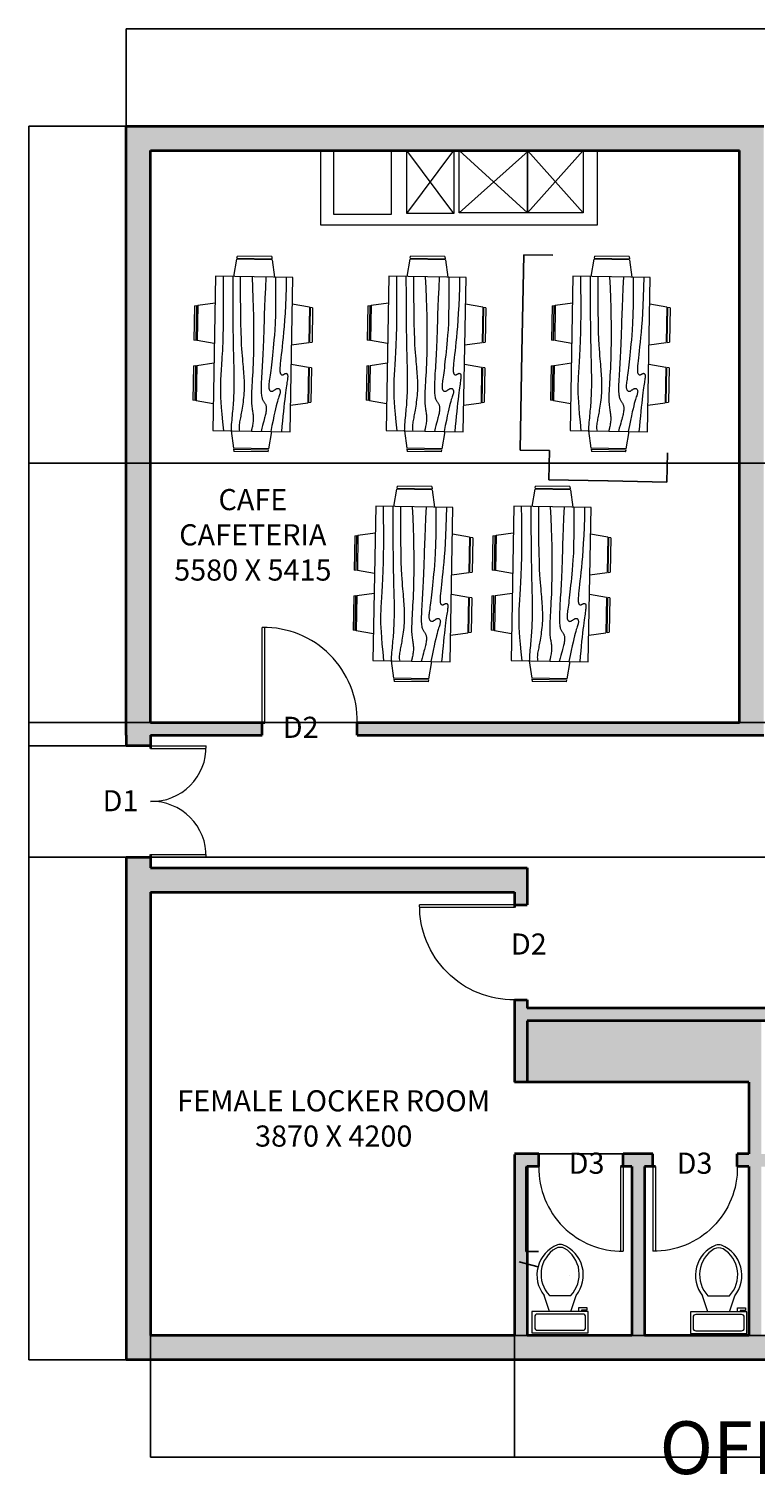
# Model space of a CAD drawing. Units: millimetres. Extents: x 14737 to 34075, y 1723 to 15415.
# Tile 1 of 2: x 14737 to 21616, y 1723 to 15415. Entities that reach past the tile are written whole.
import ezdxf

# ---------------------------------------------------------------- set-up
doc = ezdxf.new("R2010")
doc.units = ezdxf.units.MM
doc.header["$PDMODE"] = 32
doc.header["$PDSIZE"] = 100
for name, color, linetype, lineweight in [('A-ANNO-DIMS', 2, 'Continuous', 18), ('A-ANNO-TITL', 7, 'Continuous', 35), ('A-AREA-IDEN', 7, 'Continuous', 25), ('A-DOOR', 4, 'Continuous', 18), ('A-DOOR-IDEN', 3, 'Continuous', 18), ('A-EQPM', 8, 'Continuous', 18), ('A-FLOR-FIXT', 9, 'Continuous', 18), ('A-FURN', 8, 'Continuous', 18), ('A-WALL', 7, 'Continuous', 35), ('A-WALL-PATT', 252, 'Continuous', 13)]:
    doc.layers.add(name, color=color, linetype=linetype, lineweight=lineweight)
doc.styles.get("Standard").update_dxf_attribs({"font": 'arial.ttf'})
doc.dimstyles.get("Standard").update_dxf_attribs({"dimtxt": 0.18, "dimasz": 0.18, "dimexe": 0.18, "dimexo": 0.0625, "dimgap": 0.09, "dimtad": 0, "dimtih": 1, "dimtoh": 1, "dimdec": 4, "dimzin": 0, "dimdsep": 46, "dimtxsty": 'Standard', "dimcen": 0.09, "dimadec": 0, "dimazin": 0, "dimtfac": 1, "dimtdec": 4, "dimtofl": 0, "dimtmove": 0, "dimatfit": 3, "dimfxl": 1, "dimtolj": 1, "dimtzin": 0, "dimarcsym": 0})

# ---------------------------------------------------------------- blocks, each defined once
blk = doc.blocks.new('Dining Set - 36 x 72 in.')
for p, q in [((-22, 27.5), (-22.15620000000001, 26.50042)), ((-22, 27.5), (-6, 27.5)), ((-5.843700000000012, 26.49966), (-6, 27.5)), ((6, 27.5), (5.843799999999987, 26.50042)), ((6, 27.5), (22, 27.5)), ((22.15629999999999, 26.49966), (22, 27.5)), ((-22.23430000000002, 26.00059), (-23.48470000000003, 17.99762)), ((-22.23040000000003, 26), (-5.760800000000017, 26)), ((-5.841600000000028, 26.5), (-22.15340000000003, 26.5)), ((-4.515199999999992, 17.99762), (-5.765500000000031, 25.99926)), ((5.765699999999981, 26.00059), (4.515299999999967, 17.99762)), ((5.769599999999968, 26), (22.23919999999998, 26)), ((22.15839999999997, 26.5), (5.846599999999966, 26.5)), ((23.48480000000001, 17.99762), (22.23449999999997, 25.99926)), ((36, 18), (-36, 18)), ((-36, 18), (-36, -18)), ((36, -18), (36, 18)), ((-45.49999999999999, 8.000000000000004), (-44.50040000000001, 8.156170000000007)), ((-45.49999999999999, 8.000000000000004), (-45.49999999999999, -7.999999999999996)), ((-44.5, -8.15843), (-44.5, 8.153380000000002)), ((-44.00060000000002, 8.234280000000002), (-35.99760000000003, 9.484740000000006)), ((-44, 8.230410000000003), (-44, -8.239149999999999)), ((44.00059999999996, 8.234280000000002), (35.99759999999998, 9.484740000000006)), ((44, 8.230410000000003), (44, -8.239149999999999)), ((44.5, -8.15843), (44.5, 8.153380000000002)), ((45.49999999999999, 8.000000000000004), (44.50049999999999, 8.156170000000007)), ((45.49999999999999, 8.000000000000004), (45.49999999999999, -7.999999999999996)), ((-44.49970000000002, -8.156309999999994), (-45.49999999999999, -7.999999999999996)), ((-35.99760000000003, -9.484759999999998), (-43.9993, -8.234499999999993)), ((35.99759999999998, -9.484759999999998), (43.9993, -8.234499999999993)), ((44.49969999999995, -8.156309999999994), (45.49999999999999, -7.999999999999996)), ((-36, -18), (36, -18)), ((-22.23430000000002, -26.0006), (-23.48470000000003, -17.99762)), ((-4.515199999999992, -17.99762), (-5.765500000000031, -25.99928)), ((5.765699999999981, -26.0006), (4.515299999999967, -17.99762)), ((23.48480000000001, -17.99762), (22.23449999999997, -25.99928)), ((-22.23040000000003, -26), (-5.760800000000017, -26)), ((-22, -27.5), (-22.15620000000001, -26.50044)), ((-5.841600000000028, -26.5), (-22.15340000000003, -26.5)), ((-5.843700000000012, -26.49967), (-6, -27.5)), ((5.769599999999968, -26), (22.23919999999998, -26)), ((6, -27.5), (5.843799999999987, -26.50044)), ((22.15839999999997, -26.5), (5.846599999999966, -26.5)), ((22.15629999999999, -26.49967), (22, -27.5)), ((-22, -27.5), (-6, -27.5)), ((6, -27.5), (22, -27.5))]:
    blk.add_line(p, q)
for points in [[(-36, 15), (-31.17720000000003, 14.97754), (-26.80790000000002, 14.91406), (-22.85380000000003, 14.81543), (-19.27600000000001, 14.6875), (-16.03620000000001, 14.53613), (-13.09570000000002, 14.36718), (-10.41590000000002, 14.18652), (-7.958300000000008, 14), (-5.690400000000011, 13.81315), (-3.603499999999996, 13.63021), (-1.695400000000006, 13.45508), (0.0364999999999896, 13.29166), (1.594499999999982, 13.14388), (2.981099999999969, 13.01562), (4.198800000000005, 12.9108), (5.25, 12.83333), (6.139299999999991, 12.78613), (6.880200000000002, 12.76823), (7.488299999999981, 12.77767), (7.979199999999991, 12.8125), (8.368499999999983, 12.87077), (8.671899999999994, 12.95052), (8.904899999999998, 13.0498), (9.083300000000008, 13.16666), (9.220499999999959, 13.29899000000001), (9.32159999999999, 13.44401), (9.389499999999998, 13.59879), (9.427099999999996, 13.76041), (9.437299999999993, 13.92594), (9.423200000000008, 14.09245), (9.387499999999989, 14.257), (9.333300000000008, 14.41666), (9.263800000000003, 14.56917), (9.183600000000013, 14.71484), (9.097499999999968, 14.85465), (9.010400000000004, 14.98958), (8.92719999999997, 15.12060000000001), (8.852899999999975, 15.2487), (8.79219999999998, 15.37483), (8.75, 15.5), (8.730500000000006, 15.62467), (8.734399999999994, 15.74739), (8.761699999999962, 15.86621), (8.8125, 15.97916), (8.886699999999962, 16.08431), (8.984399999999994, 16.17968), (9.105500000000006, 16.26334), (9.25, 16.33333), (9.418900000000008, 16.38802), (9.617199999999968, 16.42708), (9.850599999999986, 16.45052), (10.125, 16.45833), (10.44630000000001, 16.45052), (10.82029999999997, 16.42708), (11.25290000000001, 16.38802), (11.75, 16.33333), (12.3184, 16.26318), (12.96940000000001, 16.17838), (13.7151, 16.07991), (14.5677, 15.96875), (15.53949999999997, 15.84586), (16.64259999999996, 15.71224), (17.88929999999999, 15.56884), (19.29169999999999, 15.41666), (20.85899999999998, 15.25667), (22.58789999999999, 15.08984), (24.47210000000001, 14.91715), (26.5052, 14.73958), (28.68090000000001, 14.5581), (30.99289999999996, 14.3737), (33.43469999999996, 14.18733), (36, 14)], [(-36, 10), (-28.97660000000002, 10.14274000000001), (-23.17250000000001, 10.20442), (-18.42410000000001, 10.19775), (-14.5677, 10.13541), (-11.43990000000002, 10.03011), (-8.87700000000001, 9.894530000000007), (-6.715399999999988, 9.741370000000005), (-4.791699999999991, 9.58333), (-2.96980000000002, 9.43082), (-1.224600000000009, 9.285150000000005), (0.4414999999999623, 9.14534), (2.02600000000001, 9.010410000000004), (3.526599999999973, 8.879390000000004), (4.940799999999967, 8.751300000000004), (6.265999999999962, 8.625160000000005), (7.5, 8.500000000000004), (8.641099999999994, 8.375490000000003), (9.691399999999987, 8.253900000000005), (10.65379999999999, 8.13818), (11.53120000000001, 8.031250000000004), (12.32669999999996, 7.936030000000005), (13.043, 7.85547), (13.68309999999997, 7.792480000000001), (14.25, 7.750000000000003), (14.74709999999999, 7.730300000000003), (15.17969999999997, 7.733070000000001), (15.55369999999999, 7.757320000000003), (15.875, 7.80208), (16.14940000000001, 7.866370000000006), (16.38279999999997, 7.94922), (16.58109999999999, 8.04964), (16.75, 8.166660000000004), (16.89439999999996, 8.29915), (17.01429999999999, 8.445310000000003), (17.1089, 8.603190000000001), (17.17709999999999, 8.77083), (17.21799999999996, 8.946290000000001), (17.2305, 9.127600000000005), (17.21369999999996, 9.312820000000006), (17.16669999999999, 9.500000000000004), (17.08949999999999, 9.687500000000004), (16.98699999999996, 9.875000000000004), (16.86489999999998, 10.0625), (16.72919999999999, 10.25), (16.5856, 10.4375), (16.44009999999997, 10.625), (16.29849999999999, 10.8125), (16.16669999999999, 11), (16.05000000000001, 11.18733), (15.95179999999999, 11.3737), (15.8752, 11.5581), (15.8229, 11.73958), (15.798, 11.91715), (15.80340000000001, 12.08984), (15.84199999999998, 12.25667), (15.91669999999999, 12.41666), (16.02949999999998, 12.56836), (16.17840000000001, 12.70833), (16.3605, 12.83268), (16.5729, 12.9375), (16.8127, 13.01888000000001), (17.07679999999999, 13.07291), (17.36250000000001, 13.0957), (17.66669999999999, 13.08333), (17.98939999999999, 13.03312), (18.34179999999998, 12.94726), (18.7382, 12.82918), (19.1927, 12.68229), (19.71949999999998, 12.51001), (20.33269999999999, 12.31575), (21.04649999999998, 12.10294), (21.875, 11.875), (22.83569999999997, 11.63354), (23.95900000000001, 11.37304), (25.27859999999999, 11.08618), (26.82819999999998, 10.76562), (28.64139999999998, 10.40405), (30.75200000000001, 9.994140000000005), (33.1936, 9.528560000000002), (36, 9.000000000000004)], [(-36, 5.500000000000003), (-30.71570000000003, 5.334800000000004), (-26.06900000000002, 5.20963), (-21.99459999999999, 5.11767), (-18.42709999999999, 5.05208), (-15.30090000000001, 5.006020000000003), (-12.55080000000004, 4.972650000000005), (-10.1112, 4.945150000000001), (-7.916699999999991, 4.916660000000003), (-5.908999999999991, 4.881670000000003), (-4.058600000000012, 4.839840000000005), (-2.342899999999985, 4.792150000000003), (-0.7395999999999959, 4.73958), (0.7738999999999692, 4.683100000000006), (2.21999999999997, 4.623700000000003), (3.621299999999962, 4.562330000000006), (5, 4.500000000000003), (6.37299999999999, 4.437820000000005), (7.734399999999993, 4.377600000000004), (9.072299999999984, 4.321290000000001), (10.375, 4.27083), (11.63089999999999, 4.228190000000001), (12.8281, 4.195310000000002), (13.95509999999996, 4.17415), (15, 4.166660000000003), (15.95400000000001, 4.174480000000006), (16.81899999999996, 4.197910000000003), (17.6001, 4.236980000000006), (18.30209999999999, 4.291660000000003), (18.92989999999997, 4.361980000000006), (19.48829999999998, 4.447910000000003), (19.98230000000001, 4.549480000000006), (20.41669999999999, 4.666660000000003), (20.79689999999999, 4.798990000000006), (21.1302, 4.944010000000002), (21.42449999999997, 5.098790000000004), (21.6875, 5.260410000000003), (21.92709999999999, 5.42594), (22.15109999999999, 5.592450000000003), (22.36719999999997, 5.757000000000001), (22.58339999999998, 5.916660000000003), (22.80649999999997, 6.068680000000004), (23.04039999999998, 6.210930000000001), (23.28789999999998, 6.341470000000004), (23.5521, 6.45833), (23.83580000000001, 6.559570000000004), (24.142, 6.643230000000006), (24.4735, 6.707350000000001), (24.83339999999998, 6.750000000000003), (25.2235, 6.76969), (25.642, 6.766920000000002), (26.08580000000001, 6.74267), (26.5521, 6.697910000000003), (27.03789999999998, 6.633620000000004), (27.54039999999998, 6.550780000000006), (28.05649999999997, 6.450360000000006), (28.58339999999998, 6.33333), (29.12419999999997, 6.19987), (29.70709999999997, 6.046870000000001), (30.36609999999996, 5.870440000000005), (31.1354, 5.666660000000003), (32.04929999999996, 5.431640000000005), (33.142, 5.161460000000001), (34.44749999999999, 4.852210000000003), (36, 4.500000000000003)], [(-36, -0.9999999999999964), (-30.79150000000004, -0.6590999999999987), (-26.01949999999999, -0.3821599999999954), (-21.65190000000001, -0.1628399999999992), (-17.65629999999999, 0.0052100000000017), (-14.00049999999999, 0.1283300000000018), (-10.65230000000002, 0.2128900000000051), (-7.579600000000027, 0.2652200000000029), (-4.75, 0.2916600000000038), (-2.134000000000014, 0.2979300000000045), (0.2878000000000043, 0.287110000000002), (2.5317, 0.2616300000000002), (4.614599999999995, 0.2239600000000017), (6.552899999999965, 0.1765100000000039), (8.363299999999981, 0.1217400000000062), (10.06229999999999, 0.0620900000000013), (11.66669999999999, 3.6e-15), (13.18989999999996, -0.0620099999999972), (14.63409999999999, -0.1210999999999949), (15.9982, -0.174319999999998), (17.28129999999999, -0.2187499999999964), (18.48230000000001, -0.2514699999999941), (19.6003, -0.2695299999999996), (20.6343, -0.2700199999999988), (21.58339999999999, -0.2499999999999964), (22.44810000000001, -0.2076799999999999), (23.23570000000001, -0.1458399999999962), (23.95490000000001, -0.0683599999999949), (24.6146, 0.0208300000000001), (25.2235, 0.1178400000000046), (25.79039999999998, 0.2187500000000035), (26.32409999999999, 0.3196600000000025), (26.83339999999998, 0.4166600000000038), (27.32650000000001, 0.5061800000000041), (27.80989999999997, 0.5859300000000012), (28.2894, 0.6539700000000046), (28.77089999999999, 0.7083300000000002), (29.26009999999997, 0.7470700000000045), (29.76299999999998, 0.7682300000000062), (30.28550000000001, 0.7698500000000017), (30.83339999999998, 0.7500000000000036), (31.40879999999999, 0.707840000000001), (31.99939999999998, 0.6471300000000006), (32.589, 0.5727500000000028), (33.16149999999999, 0.4895800000000002), (33.70079999999996, 0.402500000000007), (34.19079999999997, 0.3164000000000051), (34.61529999999999, 0.2361600000000017), (34.95839999999998, 0.1666600000000038), (35.20990000000001, 0.1116500000000009), (35.38479999999998, 0.0703100000000028), (35.50399999999996, 0.0406900000000015), (35.58859999999999, 0.0208300000000001), (35.65940000000001, 0.0087900000000012), (35.73769999999996, 0.0026000000000046), (35.8442, 0.0003200000000056), (36, 3.6e-15)], [(-36, -6.499999999999996), (-27.18430000000001, -6.312669999999993), (-20.084, -6.126299999999996), (-14.46899999999999, -5.941899999999993), (-10.10939999999999, -5.760419999999999), (-6.77520000000004, -5.582849999999996), (-4.236300000000028, -5.410159999999994), (-2.262900000000001, -5.243329999999996), (-0.625, -5.083339999999996), (0.8707999999999742, -4.930989999999997), (2.271500000000003, -4.786459999999994), (3.587199999999995, -4.649739999999997), (4.828100000000006, -4.520839999999996), (6.004599999999982, -4.399739999999997), (7.127000000000009, -4.286459999999994), (8.205299999999966, -4.180989999999997), (9.25, -4.083339999999996), (10.27049999999997, -3.993819999999995), (11.27339999999998, -3.914069999999998), (12.2647, -3.846029999999995), (13.25, -3.791669999999999), (14.23539999999997, -3.752929999999995), (15.22659999999996, -3.731769999999993), (16.22949999999997, -3.730149999999998), (17.25, -3.749999999999996), (18.2912, -3.792479999999994), (19.3451, -3.855469999999993), (20.40089999999998, -3.936039999999994), (21.4479, -4.031249999999996), (22.47539999999998, -4.138189999999998), (23.47269999999998, -4.253909999999994), (24.4289, -4.375489999999995), (25.33339999999999, -4.499999999999996), (26.17849999999999, -4.624919999999999), (26.96940000000001, -4.749349999999996), (27.71449999999999, -4.872809999999997), (28.4219, -4.994789999999998), (29.09999999999996, -5.114829999999994), (29.75720000000001, -5.232419999999994), (30.40159999999997, -5.347089999999997), (31.04169999999999, -5.458339999999996), (31.68369999999999, -5.564369999999993), (32.32619999999997, -5.658209999999993), (32.9658, -5.731529999999995), (33.59899999999999, -5.776039999999998), (34.22239999999999, -5.783449999999998), (34.83269999999999, -5.745449999999994), (35.4264, -5.653729999999999), (36, -5.499999999999996)], [(-36, -9.999999999999996), (-26.40219999999999, -9.812989999999996), (-18.46750000000003, -9.628909999999994), (-11.9839, -9.450689999999998), (-6.739599999999995, -9.281249999999996), (-2.522600000000011, -9.123539999999995), (0.8788999999999872, -8.980469999999993), (3.676899999999989, -8.854979999999994), (6.083300000000008, -8.749999999999996), (8.276700000000005, -8.667649999999998), (10.30209999999999, -8.606769999999994), (12.1712, -8.565429999999996), (13.89580000000001, -8.54167), (15.48759999999998, -8.533529999999995), (16.95830000000001, -8.539069999999999), (18.31970000000001, -8.556319999999994), (19.58339999999998, -8.583339999999996), (20.76159999999999, -8.618409999999994), (21.86849999999998, -8.660809999999994), (22.91879999999998, -8.710039999999996), (23.9271, -8.765629999999998), (24.90809999999999, -8.827069999999996), (25.87629999999996, -8.89388), (26.84649999999999, -8.96558), (27.83339999999999, -9.04167), (28.84739999999999, -9.121179999999997), (29.88279999999998, -9.201169999999994), (30.93000000000001, -9.278239999999993), (31.97919999999999, -9.348959999999995), (33.02049999999997, -9.409909999999998), (34.04429999999996, -9.45768), (35.04069999999996, -9.488849999999996), (36, -9.499999999999996)], [(-36, -14.5), (-30.0881, -14.33512999999999), (-25.03320000000002, -14.21224), (-20.7312, -14.12646999999999), (-17.0781, -14.07292), (-13.97000000000003, -14.04670999999999), (-11.30270000000001, -14.04296999999999), (-8.972399999999993, -14.05680999999999), (-6.875, -14.08333999999999), (-4.922400000000038, -14.11832999999999), (-3.09050000000002, -14.16015999999999), (-1.370900000000006, -14.20784999999999), (0.2447999999999979, -14.26042), (1.764700000000004, -14.31689999999999), (3.197299999999984, -14.37629999999999), (4.550700000000006, -14.43766999999999), (5.833300000000008, -14.5), (7.055399999999963, -14.5621), (8.235000000000014, -14.62174999999999), (9.392200000000003, -14.67652), (10.54689999999999, -14.72395999999999), (11.7192, -14.76164), (12.92899999999997, -14.78711), (14.19649999999996, -14.79794), (15.54169999999999, -14.79167), (16.99329999999998, -14.76423999999999), (18.61519999999996, -14.70508), (20.48039999999998, -14.60197), (22.66149999999999, -14.44270999999999), (25.2312, -14.21509), (28.26240000000002, -13.90689999999999), (31.8277, -13.50594), (36, -13)]]:
    blk.add_lwpolyline(points)
blk = doc.blocks.new('Toilet - top')
for p, q in [((9.5, -6), (9.5, -2)), ((-10, -8.5), (-8, -8.5)), ((-10, -9.5), (-10, -8.5)), ((-7, -9.5), (-10, -9.5)), ((-8, -8.5), (-8, -8)), ((-7, -8), (-7, -9.5)), ((-4, -8), (-6, -14)), ((4, -8), (6, -14)), ((4, -14), (-4, -14))]:
    blk.add_line(p, q)
blk.add_lwpolyline([(10.5, -8), (10.5, 0), (-10.5, 0), (-10.5, -8)], close=True)
for points in [[(-9.5, -2), (-9.5, -6)], [(8.5, -1), (-8.5, -1)], [(-8.5, -7), (8.5, -7)]]:
    blk.add_lwpolyline(points)
for centre, radius, start, end in [((-8.625, -1.875), 0.8838834999999999, 81.86989999999999, 188.1301), ((8.625, -1.875), 0.8838834999999999, 351.8699, 98.13009999999998), ((-8.625, -6.125), 0.8838834999999999, 171.869898, 278.1301), ((8.625, -6.125), 0.8838834999999999, 261.8699, 8.130099999999993), ((3.519562435188956, -21.58049502388982), 12.16902005083646, 141.4691096810948, 247.9714346835576), ((4.199957580658807, -21.81740929088453), 11.3291791325804, 136.3677254423718, 238.946823937405), ((-3.519499936778316, -21.58047137067522), 12.16903423757823, 292.0284332733152, 38.53070636800453), ((-4.199890672038477, -21.81738596564128), 11.32918622148567, 301.0530065773863, 43.63209216694732), ((2.09660981727e-05, -27.87646475467881), 4, 245.7318247449371, 294.2681740488959), ((2.09415214183e-05, -28.99996806116075), 4, 254.8605283244437, 285.1394707718433)]:
    blk.add_arc(centre, radius, start, end)
blk = doc.blocks.new('DOOR-D2-900')
for p, q in [((-3.638e-12, 0), (-3.638e-12, 900)), ((25.39999999999782, 0), (25.39999999999782, 900))]:
    blk.add_line(p, q)
blk.add_arc((12.69999999999709, 12.69999999999891), 887.3908834330009, 359.1799766532175, 90.82002334678252)
blk = doc.blocks.new('DOOR-D3-800')
for p, q in [((774.702568529894, 800.102568529895), (774.702568529894, 0.1025685298941426)), ((800.1025685298955, 800.102568529895), (800.1025685298955, 0.1025685298941426))]:
    blk.add_line(p, q)
blk.add_arc((787.4025685298947, 787.4025685298961), 787.4024257011142, 179.0758372986705, 270.9241627013018)
blk = doc.blocks.new('*D8')
at = {"layer": 'A-ANNO-DIMS', "color": 0, "lineweight": -2, "transparency": 16777216}
for p, q in [((19424.11609662125, 13276.55799013177), (19407.63221019421, 12352.18715055539)), ((19701.47698006667, 13271.79196776401), (19423.93933458261, 13276.74117086683)), ((19391.1417945735, 11427.45017182486), (19407.62568100054, 12351.82101140123)), ((19668.4962593225, 11422.3242066834), (19390.95861383844, 11427.27340978622))]:
    blk.add_line(p, q, dxfattribs=at)
at = {"layer": 'A-ANNO-DIMS', "color": 0, "transparency": 16777216}
for points in [[(19424.08610139011, 13276.55852502314), (19424.14609185239, 13276.5574552404), (19424.11930596946, 13276.73796151862)], [(19391.11179934236, 11427.45070671622), (19391.17178980464, 11427.44963693349), (19391.13858522529, 11427.27020043801)]]:
    blk.add_solid(points, dxfattribs=at)
at = {"layer": 'Defpoints', "color": 0, "transparency": 16777216}
for p in [(19701.53947013155, 13271.79085340699), (19391.13858522529, 11427.27020043801), (19668.55874938738, 11422.32309232638)]:
    blk.add_point(p, dxfattribs=at)
at = {"layer": 'A-ANNO-DIMS', "color": 0, "transparency": 16777216, "insert": (19407.62894559737, 12352.00408097831), "char_height": 0.18, "attachment_point": 5}
blk.add_mtext('\\A1;DINING SET 1850 TYP.', dxfattribs=at)
blk = doc.blocks.new('*D9')
at = {"layer": 'A-ANNO-DIMS', "color": 0, "lineweight": -2, "transparency": 16777216}
for p, q in [((19668.55763503035, 11422.2606022615), (19663.60843192753, 11144.72295677744)), ((20786.36782029886, 11402.32719961392), (20781.41861719604, 11124.78955412986)), ((19663.79161266259, 11144.89971881608), (20221.85726597002, 11134.94798683352)), ((20781.2418551574, 11124.97273486492), (20223.17620184997, 11134.92446684748))]:
    blk.add_line(p, q, dxfattribs=at)
at = {"layer": 'A-ANNO-DIMS', "color": 0, "transparency": 16777216}
for points in [[(19663.79214755396, 11144.92971404722), (19663.79107777122, 11144.86972358494), (19663.61164127574, 11144.90292816429)], [(20781.24239004877, 11125.00273009606), (20781.24132026603, 11124.94273963378), (20781.42182654425, 11124.96952551671)]]:
    blk.add_solid(points, dxfattribs=at)
at = {"layer": 'Defpoints', "color": 0, "transparency": 16777216}
for p in [(19668.55874938737, 11422.32309232638), (20786.36893465588, 11402.3896896788), (20781.42182654425, 11124.96952551671)]:
    blk.add_point(p, dxfattribs=at)
at = {"layer": 'A-ANNO-DIMS', "color": 0, "transparency": 16777216, "insert": (20222.51673391, 11134.9362268405), "char_height": 0.18, "attachment_point": 5}
blk.add_mtext('\\A1;1118 TYP.', dxfattribs=at)
blk = doc.blocks.new('*D14')
at = {"layer": 'A-ANNO-DIMS', "color": 0, "lineweight": -2, "transparency": 16777216}
for p, q in [((19564.08164650023, 4643.424739033563), (19443.44825288388, 4643.424739033563)), ((19443.62825288388, 4643.244739033563), (19443.62825288388, 4241.887058175034)), ((19443.62825288388, 3840.165448257842), (19443.62825288388, 4241.52312911637)), ((19564.08164650023, 3839.985448257844), (19443.44825288388, 3839.985448257843))]:
    blk.add_line(p, q, dxfattribs=at)
at = {"layer": 'A-ANNO-DIMS', "color": 0, "transparency": 16777216}
for points in [[(19443.59825288388, 4643.244739033563), (19443.65825288388, 4643.244739033563), (19443.62825288388, 4643.424739033563)], [(19443.59825288388, 3840.165448257842), (19443.65825288388, 3840.165448257842), (19443.62825288388, 3839.985448257843)]]:
    blk.add_solid(points, dxfattribs=at)
at = {"layer": 'Defpoints', "color": 0, "transparency": 16777216}
for p in [(19443.62825288388, 4643.424739033563), (19564.14414650023, 4643.424739033563), (19564.14414650023, 3839.985448257844)]:
    blk.add_point(p, dxfattribs=at)
at = {"layer": 'A-ANNO-DIMS', "color": 0, "transparency": 16777216, "insert": (19443.62825288387, 4241.705093645697), "char_height": 0.18, "attachment_point": 5}
blk.add_mtext('\\A1;D3 803 TYP.', dxfattribs=at)
blk = doc.blocks.new('*D15')
at = {"layer": 'A-ANNO-DIMS', "color": 0, "lineweight": -2, "transparency": 16777216}
for p, q in [((19564.14414650022, 4643.487239033561), (19564.14414650022, 4764.120632649919)), ((19564.32414650022, 4763.940632649918), (19965.26565409815, 4763.940632649918)), ((20367.40343727589, 4763.940632649918), (19966.46192967796, 4763.940632649918)), ((20367.58343727589, 4643.487239033561), (20367.58343727589, 4764.120632649919))]:
    blk.add_line(p, q, dxfattribs=at)
at = {"layer": 'A-ANNO-DIMS', "color": 0, "transparency": 16777216}
for points in [[(19564.32414650022, 4763.970632649919), (19564.32414650022, 4763.91063264992), (19564.14414650022, 4763.940632649918)], [(20367.40343727589, 4763.970632649919), (20367.40343727589, 4763.91063264992), (20367.58343727589, 4763.940632649918)]]:
    blk.add_solid(points, dxfattribs=at)
at = {"layer": 'Defpoints', "color": 0, "transparency": 16777216}
for p in [(20367.58343727589, 4763.940632649918), (19564.14414650022, 4643.424739033561), (20367.58343727589, 4643.424739033561)]:
    blk.add_point(p, dxfattribs=at)
at = {"layer": 'A-ANNO-DIMS', "color": 0, "transparency": 16777216, "insert": (19965.86379188805, 4763.940632649918), "char_height": 0.18, "attachment_point": 5}
blk.add_mtext('\\A1;803 TYP.', dxfattribs=at)
blk = doc.blocks.new('*D22')
at = {"layer": 'A-ANNO-DIMS', "color": 0, "lineweight": -2, "transparency": 16777216}
for p, q in [((15658.583437, 14493.487239), (15658.583437, 15414.604739)), ((15658.763437, 15414.424739), (24405.66253659072, 15414.424739)), ((33153.403437, 15414.424739), (24406.50433740928, 15414.424739)), ((33153.583437, 13323.487239), (33153.583437, 15414.604739))]:
    blk.add_line(p, q, dxfattribs=at)
at = {"layer": 'A-ANNO-DIMS', "color": 0, "transparency": 16777216}
for points in [[(15658.763437, 15414.454739), (15658.763437, 15414.394739), (15658.583437, 15414.424739)], [(33153.403437, 15414.454739), (33153.403437, 15414.394739), (33153.583437, 15414.424739)]]:
    blk.add_solid(points, dxfattribs=at)
at = {"layer": 'Defpoints', "color": 0, "transparency": 16777216}
for p in [(33153.583437, 15414.424739), (15658.583437, 14493.424739), (33153.583437, 13323.424739)]:
    blk.add_point(p, dxfattribs=at)
at = {"layer": 'A-ANNO-DIMS', "color": 0, "transparency": 16777216, "insert": (24406.083437, 15414.424739), "char_height": 0.18, "attachment_point": 5}
blk.add_mtext('\\A1;17495', dxfattribs=at)
blk = doc.blocks.new('*D24')
at = {"layer": 'A-ANNO-DIMS', "color": 0, "lineweight": -2, "transparency": 16777216}
for p, q in [((15658.520937, 14493.424739), (14737.40343700001, 14493.424739)), ((14737.58343700001, 14493.24473900001), (14737.58343700001, 8653.606642137793)), ((14737.58343700001, 2813.604739), (14737.58343700001, 8653.242835862213)), ((15658.520937, 2813.424739000001), (14737.40343700001, 2813.424739000001))]:
    blk.add_line(p, q, dxfattribs=at)
at = {"layer": 'A-ANNO-DIMS', "color": 0, "transparency": 16777216}
for points in [[(14737.55343700001, 14493.24473900001), (14737.61343700001, 14493.24473900001), (14737.58343700001, 14493.424739)], [(14737.55343700001, 2813.604739), (14737.61343700001, 2813.604739), (14737.58343700001, 2813.424739000001)]]:
    blk.add_solid(points, dxfattribs=at)
at = {"layer": 'Defpoints', "color": 0, "transparency": 16777216}
for p in [(14737.58343700001, 14493.424739), (15658.583437, 14493.424739), (15658.583437, 2813.424739000001)]:
    blk.add_point(p, dxfattribs=at)
at = {"layer": 'A-ANNO-DIMS', "color": 0, "transparency": 16777216, "insert": (14737.58343700001, 8653.424739), "char_height": 0.18, "attachment_point": 5}
blk.add_mtext('\\A1;11680', dxfattribs=at)
blk = doc.blocks.new('*D27')
at = {"layer": 'A-ANNO-DIMS', "color": 0, "lineweight": -2, "transparency": 16777216}
for p, q in [((27983.52093700001, 11303.424739), (14737.40343700001, 11303.424739)), ((14737.58343700001, 11303.244739), (14737.58343700001, 10076.10664213779)), ((14737.58343700001, 8848.604739000002), (14737.58343700001, 10075.74283586221)), ((27983.52093700001, 8848.424739000004), (14737.40343700001, 8848.424739000002))]:
    blk.add_line(p, q, dxfattribs=at)
at = {"layer": 'A-ANNO-DIMS', "color": 0, "transparency": 16777216}
for points in [[(14737.55343700001, 11303.244739), (14737.61343700001, 11303.244739), (14737.58343700001, 11303.424739)], [(14737.55343700001, 8848.604739000002), (14737.61343700001, 8848.604739000002), (14737.58343700001, 8848.424739000002)]]:
    blk.add_solid(points, dxfattribs=at)
at = {"layer": 'Defpoints', "color": 0, "transparency": 16777216}
for p in [(14737.58343700001, 11303.424739), (27983.58343700002, 11303.424739), (27983.58343700002, 8848.424739000004)]:
    blk.add_point(p, dxfattribs=at)
at = {"layer": 'A-ANNO-DIMS', "color": 0, "transparency": 16777216, "insert": (14737.58343700001, 10075.92473899999), "char_height": 0.18, "attachment_point": 5}
blk.add_mtext('\\A1;2455', dxfattribs=at)
blk = doc.blocks.new('*D28')
at = {"layer": 'A-ANNO-DIMS', "color": 0, "lineweight": -2, "transparency": 16777216}
for p, q in [((15888.583437, 3043.362239), (15888.583437, 1892.244739)), ((19338.583437, 3043.362239), (19338.583437, 1892.244739)), ((15888.763437, 1892.424739), (17613.22503318008, 1892.424739)), ((19338.403437, 1892.424739), (17613.94184081992, 1892.424739))]:
    blk.add_line(p, q, dxfattribs=at)
at = {"layer": 'A-ANNO-DIMS', "color": 0, "transparency": 16777216}
for points in [[(15888.763437, 1892.454739), (15888.763437, 1892.394739), (15888.583437, 1892.424739)], [(19338.403437, 1892.454739), (19338.403437, 1892.394739), (19338.583437, 1892.424739)]]:
    blk.add_solid(points, dxfattribs=at)
at = {"layer": 'Defpoints', "color": 0, "transparency": 16777216}
for p in [(15888.583437, 3043.424739), (19338.583437, 3043.424739), (19338.583437, 1892.424739)]:
    blk.add_point(p, dxfattribs=at)
at = {"layer": 'A-ANNO-DIMS', "color": 0, "transparency": 16777216, "insert": (17613.583437, 1892.424739), "char_height": 0.18, "attachment_point": 5}
blk.add_mtext('\\A1;3450', dxfattribs=at)
blk = doc.blocks.new('*D29')
at = {"layer": 'A-ANNO-DIMS', "color": 0, "lineweight": -2, "transparency": 16777216}
for p, q in [((19338.583437, 3043.362239), (19338.583437, 1892.244739)), ((24003.583437, 3043.362239), (24003.583437, 1892.244739)), ((19338.763437, 1892.424739), (21670.72036742292, 1892.424739)), ((24003.403437, 1892.424739), (21671.44650657708, 1892.424739))]:
    blk.add_line(p, q, dxfattribs=at)
at = {"layer": 'A-ANNO-DIMS', "color": 0, "transparency": 16777216}
for points in [[(19338.763437, 1892.454739), (19338.763437, 1892.394739), (19338.583437, 1892.424739)], [(24003.403437, 1892.454739), (24003.403437, 1892.394739), (24003.583437, 1892.424739)]]:
    blk.add_solid(points, dxfattribs=at)
at = {"layer": 'Defpoints', "color": 0, "transparency": 16777216}
for p in [(19338.583437, 3043.424739), (24003.583437, 3043.424739), (24003.583437, 1892.424739)]:
    blk.add_point(p, dxfattribs=at)
at = {"layer": 'A-ANNO-DIMS', "color": 0, "transparency": 16777216, "insert": (21671.083437, 1892.424739), "char_height": 0.18, "attachment_point": 5}
blk.add_mtext('\\A1;4665', dxfattribs=at)
blk = doc.blocks.new('*D30')
at = {"layer": 'A-ANNO-DIMS', "color": 0, "lineweight": -2, "transparency": 16777216}
for p, q in [((15658.520937, 8628.424739000004), (14737.40343700001, 8628.424739000004)), ((14737.58343700001, 8628.244739000002), (14737.58343700001, 8101.106642137793)), ((14737.58343700001, 7573.604739000003), (14737.58343700001, 8100.742835862213)), ((15658.520937, 7573.424739000003), (14737.40343700001, 7573.424739000003))]:
    blk.add_line(p, q, dxfattribs=at)
at = {"layer": 'A-ANNO-DIMS', "color": 0, "transparency": 16777216}
for points in [[(14737.55343700001, 8628.244739000002), (14737.61343700001, 8628.244739000002), (14737.58343700001, 8628.424739000004)], [(14737.55343700001, 7573.604739000003), (14737.61343700001, 7573.604739000003), (14737.58343700001, 7573.424739000003)]]:
    blk.add_solid(points, dxfattribs=at)
at = {"layer": 'Defpoints', "color": 0, "transparency": 16777216}
for p in [(14737.58343700001, 8628.424739000004), (15658.583437, 8628.424739000004), (15658.583437, 7573.424739000003)]:
    blk.add_point(p, dxfattribs=at)
at = {"layer": 'A-ANNO-DIMS', "color": 0, "transparency": 16777216, "insert": (14737.58343700001, 8100.924738999998), "char_height": 0.18, "attachment_point": 5}
blk.add_mtext('\\A1;1055', dxfattribs=at)
blk = doc.blocks.new('*D31')
at = {"layer": 'A-ANNO-DIMS', "color": 0, "lineweight": -2, "transparency": 16777216}
for p, q in [((15888.64593700001, 7573.424739000003), (34074.76343700003, 7573.424739000007)), ((34074.58343700003, 7573.244739000006), (34074.58343700003, 5308.606703529336)), ((34074.58343700003, 3043.604739000004), (34074.58343700003, 5308.242774470673)), ((15888.64593700001, 3043.424739000001), (34074.76343700003, 3043.424739000004))]:
    blk.add_line(p, q, dxfattribs=at)
at = {"layer": 'A-ANNO-DIMS', "color": 0, "transparency": 16777216}
for points in [[(34074.55343700003, 7573.244739000006), (34074.61343700003, 7573.244739000006), (34074.58343700003, 7573.424739000007)], [(34074.55343700003, 3043.604739000004), (34074.61343700003, 3043.604739000004), (34074.58343700003, 3043.424739000004)]]:
    blk.add_solid(points, dxfattribs=at)
at = {"layer": 'Defpoints', "color": 0, "transparency": 16777216}
for p in [(15888.58343700001, 7573.424739000003), (34074.58343700003, 7573.424739000007), (15888.58343700001, 3043.424739000001)]:
    blk.add_point(p, dxfattribs=at)
at = {"layer": 'A-ANNO-DIMS', "color": 0, "transparency": 16777216, "insert": (34074.58343700002, 5308.424738999995), "char_height": 0.18, "attachment_point": 5}
blk.add_mtext('\\A1;4530', dxfattribs=at)
blk = doc.blocks.new('*D37')
at = {"layer": 'A-ANNO-DIMS', "color": 0, "lineweight": -2, "transparency": 16777216}
for p, q in [((19380.52345272353, 3743.08269092518), (19559.71828907084, 3696.003638388706)), ((19858.75059399999, 3617.416581999999), (19858.93059399999, 3617.416582000001)), ((19858.84059399999, 3617.326582), (19858.84059399999, 3617.506581999999))]:
    blk.add_line(p, q, dxfattribs=at)
at = {"layer": 'A-ANNO-DIMS', "color": 0, "transparency": 16777216}
blk.add_solid([(19559.72591213562, 3696.032653710232), (19559.71066600606, 3695.974623067179), (19559.892381, 3695.9579)], dxfattribs=at)
at = {"layer": 'Defpoints', "color": 0, "transparency": 16777216}
for p in [(19559.892381, 3695.9579), (19858.84059399999, 3617.416582)]:
    blk.add_point(p, dxfattribs=at)
at = {"layer": 'A-ANNO-DIMS', "color": 0, "transparency": 16777216, "insert": (19379.86748410143, 3743.082690925179), "char_height": 0.18, "attachment_point": 5}
blk.add_mtext('\\A1;8X R309.1', dxfattribs=at)

msp = doc.modelspace()

# ---------------------------------------------------------------- hatches: boundary and pattern name
at = {"layer": 'A-WALL-PATT'}
h = msp.add_hatch(color=256, dxfattribs=at)
h.dxf.hatch_style = 1
h.paths.add_polyline_path([(15888.58343727589, 14263.42473903341), (21468.58343727589, 14263.42473903341), (21468.58343727589, 8848.424739033417), (17848.13203580986, 8848.424739033413), (17848.13203580986, 8728.424739033415), (21698.58343727589, 8728.424739033415), (21698.58343727589, 14493.42473903341), (15658.58343727589, 14493.42473903341), (15658.58343727589, 8728.424739033415), (15658.58343727589, 8628.424739033413), (15888.58343727588, 8628.424739033413), (15888.58343727588, 8728.424739033415), (16948.13203580987, 8728.424739033415), (16948.13203580987, 8848.424739033413), (15888.58343727589, 8848.424739033413)])
h.paths.add_polyline_path([(33153.58343727589, 13323.42473903341), (27983.58343727589, 13323.42473903341), (24480.16591345426, 13323.42473903341), (24480.16591345426, 13093.42473903341), (27983.58343727589, 13093.42473903341), (27983.58343727589, 11423.42473903341), (23613.58343727589, 11423.42473903341), (23613.58343727589, 13323.42473903341), (23493.58343727589, 13323.42473903341), (23493.58343727589, 11303.42473903341), (24208.58343727589, 11303.42473903341), (24208.58343727589, 9367.011203696671), (24208.58343727589, 8728.424739033415), (24558.5834372759, 8728.424739033411), (24558.5834372759, 8848.424739033413), (24438.5834372759, 8848.424739033413), (24438.5834372759, 11303.42473903341), (27983.58343727589, 11303.42473903341), (27983.58343727589, 8848.42473903341), (25458.58343727589, 8848.424739033413), (25458.58343727589, 8728.424739033411), (27873.58343727589, 8728.42473903341), (27873.58343727589, 8628.424739033413), (28103.58343727589, 8628.424739033413), (28103.58343727589, 8728.42473903341), (28223.58343727589, 8728.42473903341), (28223.58343727589, 8848.424739033408), (28103.58343727589, 8848.42473903341), (28103.58343727589, 13093.42473903341), (32923.58343727589, 13093.42473903341), (32923.5834372759, 8848.42473903341), (29123.58343727589, 8848.424739033408), (29123.58343727589, 8728.42473903341), (32923.58343727589, 8728.42473903341), (32923.58343727589, 3043.424739033409), (28103.58343727589, 3043.424739033409), (28103.58343727589, 7573.424739033412), (27873.58343727589, 7573.424739033412), (27873.58343727589, 7473.424739033409), (23773.5834372759, 7473.424739033409), (23773.58343727589, 7123.424739033409), (24003.5834372759, 7123.424739033409), (24003.5834372759, 7243.424739033409), (27873.58343727589, 7243.424739033409), (27873.58343727589, 3043.424739033409), (24003.58343727589, 3043.42473903341), (24003.58343727589, 4763.42473903341), (23664.58343727588, 4763.42473903341), (23664.58343727588, 4643.424739033411), (23773.58343727589, 4643.42473903341), (23773.58343727589, 3043.424739033409), (22784.58343727589, 3043.424739033409), (22784.58343727588, 4643.42473903341), (22864.58343727588, 4643.424739033411), (22864.58343727588, 4763.424739033409), (22584.58343727588, 4763.424739033409), (22584.58343727588, 4643.424739033409), (22664.58343727588, 4643.424739033409), (22664.58343727589, 3043.424739033409), (21675.58343727589, 3043.424739033409), (21675.58343727589, 4643.424739033409), (21784.58343727588, 4643.424739033409), (21784.58343727588, 4763.424739033409), (21675.58343727589, 4763.42473903341), (21675.58343727589, 6023.424739033409), (19458.58343727589, 6023.424739033409), (19458.58343727589, 5443.424739033409), (21556.58343727589, 5443.424739033409), (21556.58343727589, 4763.424739033409), (21447.58343727589, 4763.42473903341), (21447.58343727589, 4643.424739033409), (21556.58343727589, 4643.42473903341), (21556.58343727588, 3043.42473903341), (20567.58343727589, 3043.424739033409), (20567.58343727589, 4643.424739033409), (20647.58343727589, 4643.424739033409), (20647.58343727589, 4763.42473903341), (20367.58343727589, 4763.42473903341), (20367.58343727589, 4643.424739033409), (20447.58343727589, 4643.424739033409), (20447.58343727589, 3043.424739033409), (19458.58343727589, 3043.424739033409), (19458.58343727589, 4643.424739033409), (19567.58343727589, 4643.424739033409), (19567.58343727589, 4763.42473903341), (19338.58343727589, 4763.42473903341), (19338.58343727589, 3043.42473903341), (15888.58343727589, 3043.42473903341), (15888.58343727589, 7243.424739033411), (19338.58343727589, 7243.424739033411), (19338.58343727589, 7123.42473903341), (19458.58343727589, 7123.42473903341), (19458.58343727589, 7473.424739033409), (15888.58343727589, 7473.424739033411), (15888.58343727588, 7573.424739033412), (15658.58343727589, 7573.424739033412), (15658.58343727589, 7473.42473903341), (15658.58343727589, 2813.42473903341), (23773.58343727589, 2813.42473903341), (27873.58343727589, 2813.42473903341), (33153.58343727589, 2813.42473903341), (33153.58343727589, 8728.42473903341)])
h.paths.add_polyline_path([(24003.5834372759, 6223.424739033411), (23773.58343727589, 6223.424739033411), (23773.58343727589, 6143.42473903341), (19458.58343727589, 6143.42473903341), (19458.58343727589, 6223.42473903341), (19338.58343727589, 6223.424739033411), (19338.58343727589, 5443.42473903341), (19458.58343727589, 5443.42473903341), (19458.58343727589, 6023.424739033409), (21675.58343727589, 6023.424739033409), (23773.58343727589, 6023.424739033409), (23773.58343727589, 5443.42473903341), (24003.5834372759, 5443.42473903341)], flags=17)

# ---------------------------------------------------------------- linework, layer by layer
at = {"layer": 'A-DOOR'}
for p, q in [((15888.58343727588, 8628.424739033413), (16416.08343727589, 8628.424739033413)), ((15888.58343727588, 8603.024739033413), (16416.08343727589, 8603.024739033413)), ((15888.58343727588, 8100.924739033414), (15888.58343727588, 8100.611480549963)), ((15888.58343727589, 7598.82473903341), (16416.08343727589, 7598.82473903341)), ((15888.58343727589, 7573.424739033412), (16416.08343727589, 7573.424739033412))]:
    msp.add_line(p, q, dxfattribs=at)
for centre, start, end in [((15901.28343727588, 8615.724739033414), 268.586812670929, 1.413187329071039), ((15901.28343727588, 7585.811480549961), 358.5868126709431, 91.41318732907112)]:
    msp.add_arc(centre, 514.9566292417265, start, end, dxfattribs=at)
at = {"layer": 'A-EQPM'}
for p, q in [((18761.09281617855, 13665.94177779988), (18317.14275405541, 14263.42473903341)), ((18317.14275405541, 13665.94177779988), (18761.09281617855, 14263.42473903341)), ((19459.9030379762, 13674.15238506129), (18811.64539226104, 14263.42473903341)), ((18811.64539226104, 13674.15238506129), (19465.09031050194, 14257.61529196945)), ((19459.9030379762, 13674.15238506129), (19986.06607178595, 14263.42473903341)), ((19986.06607178595, 13674.15238506129), (19459.9030379762, 14263.42473903341))]:
    msp.add_line(p, q, dxfattribs=at)
for points in [[(17503.21844053228, 14263.42473903341), (20120.07234398981, 14263.42473903341), (20120.07234398981, 13556.31320190536), (17503.21844053228, 13556.31320190536)], [(17626.55377687244, 14263.42473903341), (18169.15945006577, 14263.42473903341), (18169.15945006577, 13657.73117053846), (17626.55377687244, 13657.73117053846)], [(18317.14275405541, 14263.42473903341), (18761.09281617855, 14263.42473903341), (18761.09281617855, 13665.94177779988), (18317.14275405541, 13665.94177779988)], [(18811.64539226104, 14263.42473903341), (19459.9030379762, 14263.42473903341), (19459.9030379762, 13674.15238506129), (18811.64539226104, 13674.15238506129)], [(19459.9030379762, 14263.42473903341), (19986.06607178595, 14263.42473903341), (19986.06607178595, 13674.15238506129), (19459.9030379762, 13674.15238506129)]]:
    msp.add_lwpolyline(points, close=True, dxfattribs=at)
at = {"layer": 'A-WALL'}
for p, q in [((15658.58343727589, 8728.424739033415), (15658.58343727589, 14493.42473903341)), ((15658.58343727589, 14493.42473903341), (21698.58343727589, 14493.42473903341)), ((15888.58343727589, 8848.424739033413), (15888.58343727589, 14263.42473903341)), ((15888.58343727589, 14263.42473903341), (21468.58343727589, 14263.42473903341)), ((21468.58343727589, 8848.424739033417), (21468.58343727589, 14263.42473903341)), ((15888.58343727589, 8848.424739033413), (16973.53203580987, 8848.424739033413)), ((16948.13203580987, 8728.424739033415), (16948.13203580987, 8848.424739033413)), ((17848.13203580986, 8728.424739033415), (17848.13203580986, 8848.424739033413)), ((17848.13203580986, 8848.424739033413), (21468.58343727589, 8848.424739033417)), ((15658.58343727589, 8728.424739033415), (15658.58343727589, 8628.424739033411)), ((15888.58343727588, 8628.424739033413), (15658.58343727589, 8628.424739033413)), ((15888.58343727588, 8728.424739033415), (16948.13203580987, 8728.424739033415)), ((15888.58343727588, 8728.424739033411), (15888.58343727588, 8603.024739033413)), ((17848.13203580986, 8728.424739033415), (21698.58343727589, 8728.424739033415)), ((15658.58343727589, 7573.424739033412), (15888.58343727589, 7573.424739033412)), ((15658.58343727589, 7573.424739033412), (15658.58343727589, 7473.42473903341)), ((15888.58343727588, 7598.82473903341), (15888.58343727589, 7473.424739033411)), ((15658.58343727589, 7473.42473903341), (15658.58343727589, 2813.42473903341)), ((15888.58343727589, 7473.424739033411), (19458.58343727589, 7473.42473903341)), ((19458.58343727589, 7473.42473903341), (19458.58343727589, 7123.42473903341)), ((15888.58343727589, 7243.424739033411), (19338.58343727589, 7243.424739033411)), ((15888.58343727589, 7243.424739033411), (15888.58343727589, 3043.424739033409)), ((19338.58343727589, 7243.424739033411), (19338.58343727589, 7098.024739033409)), ((19338.58343727589, 7123.42473903341), (19458.58343727589, 7123.42473903341)), ((19338.58343727589, 6223.42473903341), (19458.58343727589, 6223.42473903341)), ((19338.58343727589, 6223.42473903341), (19338.58343727589, 5443.424739033409)), ((19458.58343727589, 6223.42473903341), (19458.58343727589, 6143.42473903341)), ((23773.58343727589, 6143.42473903341), (19458.58343727589, 6143.42473903341)), ((23773.58343727589, 6023.424739033409), (19458.58343727589, 6023.424739033409)), ((19458.58343727589, 6023.42473903341), (19458.58343727589, 5443.424739033409)), ((21556.58343727589, 5443.424739033409), (19338.58343727589, 5443.424739033409)), ((21556.58343727589, 5443.424739033409), (21556.58343727589, 4763.42473903341)), ((19567.58343727589, 4763.42473903341), (19338.58343727589, 4763.42473903341)), ((19338.58343727589, 4758.621015478934), (19338.58343727589, 3043.424739033409)), ((19567.58343727589, 4643.424739033409), (19567.58343727589, 4763.42473903341)), ((20367.58343727589, 4643.424739033409), (20367.58343727589, 4763.42473903341)), ((20647.58343727589, 4763.42473903341), (20367.58343727589, 4763.42473903341)), ((20647.58343727589, 4643.424739033409), (20647.58343727589, 4763.42473903341)), ((21556.58343727589, 4763.42473903341), (21447.58343727589, 4763.42473903341)), ((21447.58343727589, 4643.424739033409), (21447.58343727589, 4763.42473903341)), ((19458.58343727589, 4643.424739033409), (19458.58343727589, 3043.424739033409)), ((19567.58343727589, 4643.424739033409), (19458.58343727589, 4643.424739033409)), ((20447.58343727589, 4643.424739033409), (20342.18343727589, 4643.424739033409)), ((20447.58343727589, 4643.424739033409), (20447.58343727589, 3043.424739033409)), ((20567.58343727589, 4643.424739033409), (20567.58343727589, 3043.424739033409)), ((20672.98343727589, 4643.424739033409), (20567.58343727589, 4643.424739033409)), ((21556.58343727589, 4643.424739033409), (21447.58343727589, 4643.424739033409)), ((21556.58343727589, 4643.424739033409), (21556.58343727589, 3043.424739033408)), ((19338.58343727589, 3043.424739033409), (15888.58343727589, 3043.424739033409)), ((20447.58343727589, 3043.424739033409), (19458.58343727589, 3043.424739033409)), ((21556.58343727589, 3043.424739033409), (20567.58343727588, 3043.424739033409)), ((23773.58343727589, 2813.42473903341), (15658.58343727589, 2813.42473903341))]:
    msp.add_line(p, q, dxfattribs=at)

# ---------------------------------------------------------------- block references
at = {"layer": 'A-DOOR'}
for name, p in [('DOOR-D2-900', (16948.13203580987, 8848.424739033413)), ('DOOR-D3-800', (19567.48086874599, 3843.322170503514))]:
    msp.add_blockref(name, p, dxfattribs=at)
at = {"layer": 'A-DOOR', "extrusion": (0, 0, -1), "zscale": -1, "rotation": 270.0000000000228}
msp.add_blockref('DOOR-D2-900', (-19338.58343727587, 7123.424739033184), dxfattribs=at)
at = {"layer": 'A-DOOR', "extrusion": (0, 0, -1), "zscale": -1}
msp.add_blockref('DOOR-D3-800', (-21447.68600580584, 3843.322170503546), dxfattribs=at)
at = {"layer": 'A-FLOR-FIXT', "xscale": 25.4, "yscale": 25.4, "zscale": 25.4, "rotation": 180}
for p in [(19769.44529564539, 3069.272609461658), (21271.02717996947, 3065.015438640257)]:
    msp.add_blockref('Toilet - top', p, dxfattribs=at)
at = {"layer": 'A-FURN', "xscale": 20.32705277837674, "yscale": 20.32705277837674, "zscale": 20.32705277837674, "rotation": 268.9783786024646}
for p in [(16857.81530973283, 12337.0902715429), (18499.38492214877, 12337.0902715429), (20243.95420239371, 12337.0902715429), (18374.77284684142, 10159.52685838657), (19683.19980702512, 10159.52685838657)]:
    msp.add_blockref('Dining Set - 36 x 72 in.', p, dxfattribs=at)

# ---------------------------------------------------------------- texts
at = {"layer": 'A-ANNO-TITL', "insert": (20711.77164831711, 2232.309858371271), "char_height": 500, "attachment_point": 1}
msp.add_mtext_dynamic_manual_height_columns('{\\fArial|b1|i0|c0|p34;OFFICE STAFF FLOOR PLAN}', width=11408.76462508039, gutter_width=12.5, heights=[0], dxfattribs=at)
at = {"layer": 'A-AREA-IDEN', "char_height": 200, "attachment_point": 1}
for s, insert in [('\\pxqc;{\\fArial|b1|i0|c0|p34;CAFE\\PCAFETERIA\\P5580 X 5415}', (14958.47646057251, 11058.4861046902)), ('\\pxqc;{\\fArial|b1|i0|c0|p34;FEMALE LOCKER ROOM\\P3870 X 4200}', (15724.35715335421, 5366.397277416179))]:
    msp.add_mtext_dynamic_manual_height_columns(s, width=3800.236613510075, gutter_width=12.5, heights=[0], dxfattribs=dict(at, insert=insert))
at = {"layer": 'A-DOOR-IDEN', "char_height": 200, "attachment_point": 1}
for s, insert in [('D2', (17142.33792904298, 8902.670006498356)), ('D1', (15435.21842974657, 8207.66793817468)), ('D2', (19302.94998805132, 6850.90126322758)), ('D3', (19850.41109099705, 4776.022181917107)), ('D3', (20872.98553667916, 4776.022181917107))]:
    msp.add_mtext_dynamic_manual_height_columns(s, width=370.9848257368431, gutter_width=12.5, heights=[0], dxfattribs=dict(at, insert=insert))

# ---------------------------------------------------------------- dimensions: what is measured, and where the dimension line sits
at = {"layer": 'A-ANNO-DIMS'}
for base, p1, p2, picture, middle in [((33153.583437, 15414.424739), (15658.583437, 14493.424739), (33153.583437, 13323.424739), '*D22', (24406.083437, 15414.424739)), ((19338.583437, 1892.424739), (15888.583437, 3043.424739), (19338.583437, 3043.424739), '*D28', (17613.583437, 1892.424739)), ((24003.583437, 1892.424739), (19338.583437, 3043.424739), (24003.583437, 3043.424739), '*D29', (21671.083437, 1892.424739))]:
    dim = msp.add_linear_dim(base=base, p1=p1, p2=p2, dimstyle='Standard', override={"dimdec": 0, "dimlfac": 1, "dimrnd": 0, "dimzin": 0, "dimdsep": 46, "dimlunit": 2}, dxfattribs=at)
    dim.commit()
    dim.dimension.update_dxf_attribs({"geometry": picture, "text_midpoint": middle})
for base, p1, p2, picture, middle in [((14737.58343700001, 14493.424739), (15658.583437, 2813.424739), (15658.583437, 14493.424739), '*D24', (14737.58343700001, 8653.424739)), ((14737.58343700001, 11303.424739), (27983.583437, 8848.424739), (27983.583437, 11303.424739), '*D27', (14737.58343700001, 10075.92473899999)), ((14737.58343700001, 8628.424739000004), (15658.583437, 7573.424739), (15658.583437, 8628.424739000002), '*D30', (14737.58343700001, 8100.924738999998)), ((34074.58343700003, 7573.424739000007), (15888.583437, 3043.424739), (15888.583437, 7573.424739), '*D31', (34074.58343700002, 5308.424738999995))]:
    dim = msp.add_linear_dim(base=base, p1=p1, p2=p2, angle=90, dimstyle='Standard', override={"dimdec": 0, "dimlfac": 1, "dimrnd": 0, "dimzin": 0, "dimdsep": 46, "dimlunit": 2}, dxfattribs=at)
    dim.commit()
    dim.dimension.update_dxf_attribs({"geometry": picture, "text_midpoint": middle})
for base, p1, p2, angle, text, picture, middle in [((19391.13858522529, 11427.27020043801), (19701.53947013154, 13271.79085340699), (19668.55874938737, 11422.32309232638), 268.9783786024646, 'DINING SET <> TYP.', '*D8', (19407.62894559737, 12352.00408097831)), ((20781.42182654425, 11124.96952551671), (19668.55874938737, 11422.32309232638), (20786.36893465588, 11402.3896896788), 358.9783786024646, '<> TYP.', '*D9', (20222.51673391, 11134.9362268405)), ((19443.62825288388, 4643.424739033563), (19564.14414650022, 3839.985448257841), (19564.14414650022, 4643.424739033561), 90, 'D3 <> TYP.', '*D14', (19443.62825288387, 4241.705093645697))]:
    dim = msp.add_linear_dim(base=base, p1=p1, p2=p2, angle=angle, text=text, dimstyle='Standard', override={"dimdec": 0, "dimlfac": 1, "dimrnd": 0, "dimzin": 0, "dimdsep": 46, "dimlunit": 2}, dxfattribs=at)
    dim.commit()
    dim.dimension.update_dxf_attribs({"geometry": picture, "text_midpoint": middle})
dim = msp.add_linear_dim(base=(20367.58343727589, 4763.940632649918), p1=(19564.14414650022, 4643.424739033561), p2=(20367.58343727589, 4643.424739033561), text='<> TYP.', dimstyle='Standard', override={"dimdec": 0, "dimlfac": 1, "dimrnd": 0, "dimzin": 0, "dimdsep": 46, "dimlunit": 2}, dxfattribs=at)
dim.commit()
dim.dimension.update_dxf_attribs({"geometry": '*D15', "text_midpoint": (19965.86379188805, 4763.940632649918)})
dim = msp.add_radius_dim(center=(19858.84059399999, 3617.416582), mpoint=(19559.892381, 3695.9579), text='8X <>', dimstyle='Standard', override={"dimdec": 1, "dimlfac": 1, "dimrnd": 0, "dimzin": 0, "dimdsep": 46, "dimlunit": 2}, dxfattribs=at)
dim.commit()
dim.dimension.update_dxf_attribs({"geometry": '*D37', "text_midpoint": (19380.52345272353, 3743.08269092518), "dimtype": 164})

doc.saveas('drawing.dxf')
